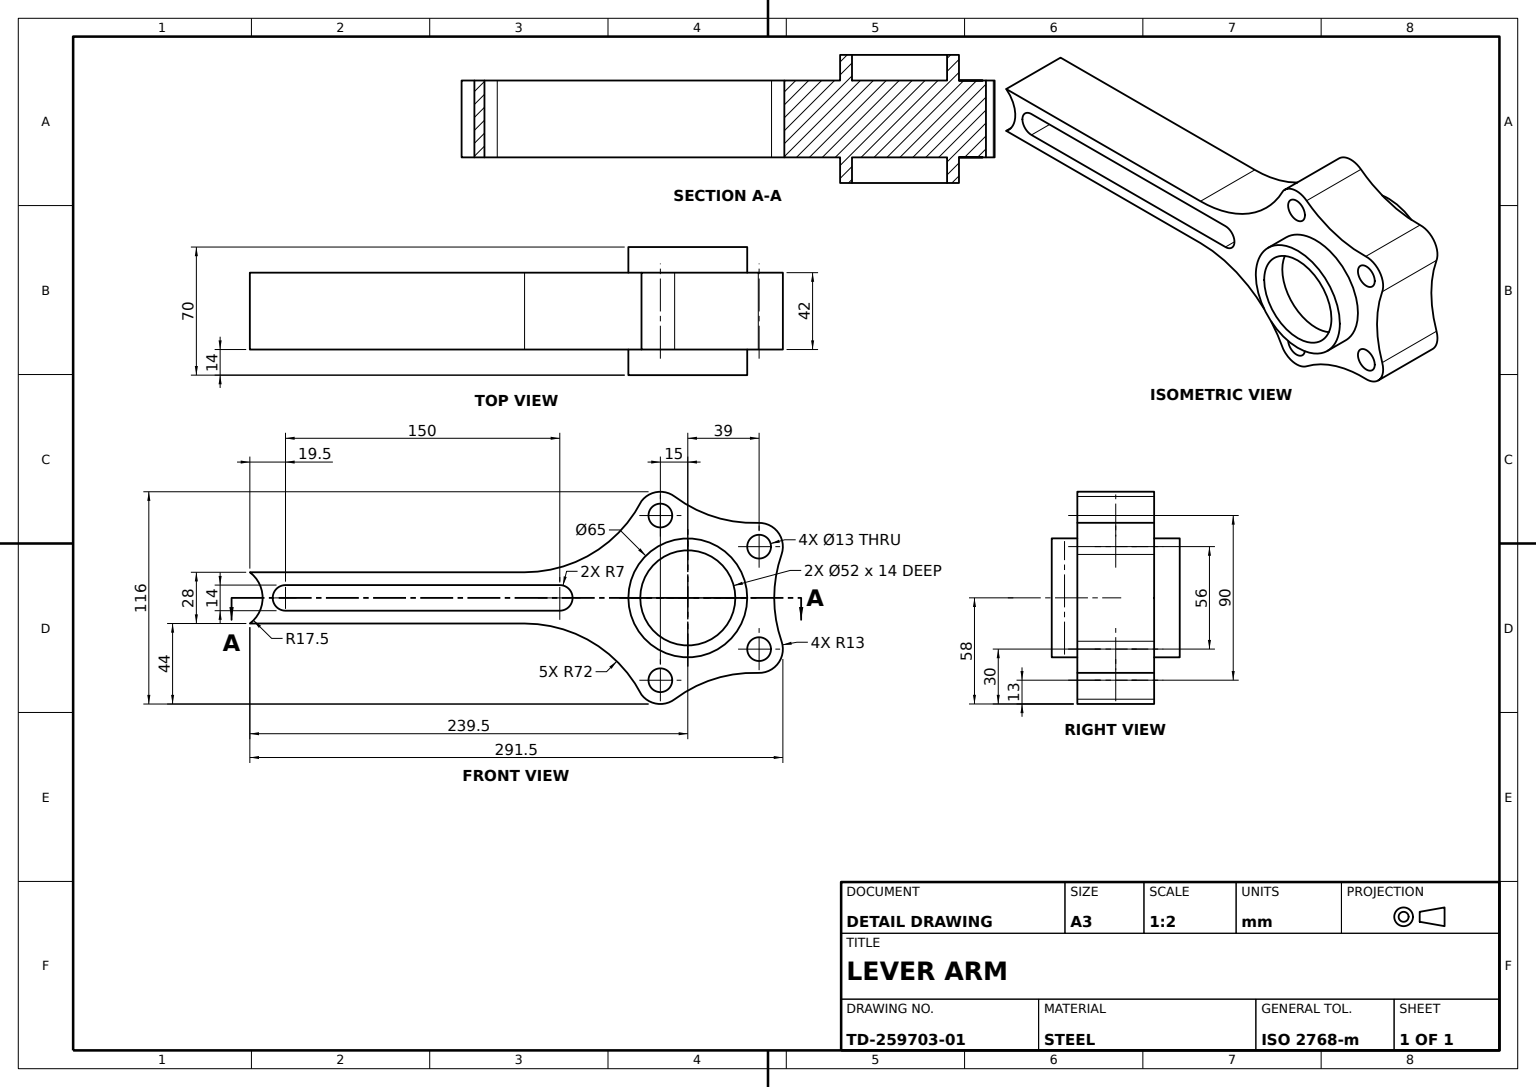
SolidWorks part; units mm, degrees
material "Plain Carbon Steel"
ref_plane "Front Plane" through (0, 0, 0) normal (0, 0, 1) x (1, 0, 0)
ref_plane "Top Plane" through (0, 0, 0) normal (0, 1, 0) x (1, 0, 0)
ref_plane "Right Plane" through (0, 0, 0) normal (1, 0, 0) x (0, 0, -1)
sketch "Hub Block Sketch" plane through (0, 0, 0) normal (0, 0, 1) x (1, 0, 0)
  line L0 (0, 76.2793) -> (0, -73.9012) construction
  line L1 (-77.1633, 0) -> (81.1425, 0) construction
  circle A4 centre (0, 0) radius 26
  circle A5 centre (0, 0) radius 32.5
  dimension "D1" = 52
  dimension "D2" = 65
extrude "Hub Block" add sketch "Hub Block Sketch" along normal mid plane 70
ref_plane "Arm Profile Plane" through (0, 0, -21) normal (0, 0, -1) x (-1, 0, 0)
sketch "Arm Profile Sketch" plane through (0, 0, -21) normal (0, 0, -1) x (-1, 0, 0)
  line L0 (0, 38.5059) -> (0, -47.9418) construction
  line L1 (89.2621, 14) -> (239.5, 14)
  line L2 (-5.6675, 45) -> (52.912, 45) construction
  line L3 (15, 30.5298) -> (15, 64.266) construction
  line L4 (15, -77.5926) -> (15, -28) construction
  line L5 (0, -45) -> (46.0324, -45) construction
  line L7 (70, 0) -> (220, 0) construction
  line L8 (70, 7) -> (220, 7)
  line L9 (70, -7) -> (220, -7)
  line L16 (55, 0) -> (256.0986, 0) construction
  line L17 (250, 4.2824) -> (250, -23.7176)
  line L19 (239.5, -14) -> (89.2621, -14)
  circle A0 centre (-39, 28) radius 6.5
  circle A1 centre (-39, -28) radius 6.5
  circle A2 centre (15, 45) radius 6.5
  circle A3 centre (15, -45) radius 6.5
  arc A4 (-38.5515, 40.9923) -> (-51.2744, 23.7176) centre (-39, 28) ccw
  arc A5 (25.3159, 52.9109) -> (7.1897, 55.3923) centre (15, 45) ccw
  arc A6 (-51.2744, -23.7176) -> (-38.5515, -40.9923) centre (-39, -28) ccw
  arc A7 (7.1897, -55.3923) -> (25.3159, -52.9109) centre (15, -45) ccw
  arc A8 (-51.2744, -23.7176) -> (-51.2744, 23.7176) centre (-119.2558, 0) ccw
  arc A9 (-38.5515, 40.9923) -> (7.1897, 55.3923) centre (-36.0674, 112.9494) ccw
  arc A13 (7.1897, -55.3923) -> (-38.5515, -40.9923) centre (-36.0674, -112.9494) ccw
  arc A26 (70, 7) -> (70, -7) centre (70, 0) ccw
  arc A27 (220, -7) -> (220, 7) centre (220, 0) ccw
  arc A28 (239.5, 14) -> (239.5, -14) centre (250, 0) ccw
  arc A30 (25.3159, 52.9109) -> (89.2621, 14) centre (89.2621, 86) ccw
  arc A31 (89.2621, -14) -> (25.3159, -52.9109) centre (89.2621, -86) ccw
  point P12 (145, 0)
  point P41 (145, 0)
  dimension "D1" = 56
  dimension "D4" = 13
  dimension "D5" = 15
  dimension "D6" = 26
  dimension "D7" = 72
  dimension "D9" = 89.2621
  dimension "D10" = 25.3159
  dimension "D15" = 70
  dimension "D11" = 4.2824
  dimension "D8" = 150
  dimension "D12" = 35
  dimension "D13" = 7
  dimension "D2" = 39
  dimension "D3" = 90
  dimension "D16" = 239.5
extrude "Arm Body" add sketch "Arm Profile Sketch" against normal blind 42 contours A31 L19 A28 L1 A30 A5 A9 A4 A8 A6 A13 A7 A27 L9 A26 L8 A3 A2 A1 A0
